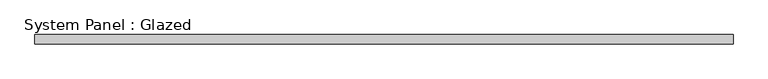
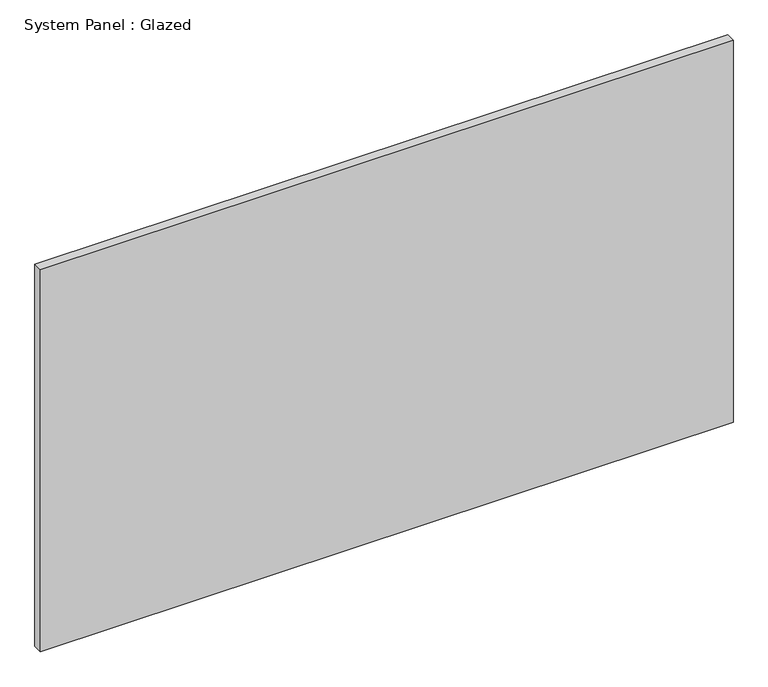
"""IFC4 building model written with IfcOpenShell, lengths in millimetres: plate geometry, System Panel : Glazed."""

from ifc_helpers import new_model, si_unit, origin, origin_with_axes, place, context, project, spatial, polyline, outline, extrude, source, transform, mapped, element, save


def system_panel_glazed_e8634194(model_context):
    return source(origin(), model_context, "Body", "SweptSolid", [
        extrude(outline(polyline([(915.0000002, 24.5), (-915.0000002, 24.5), (-915.0000002, 49.5), (915.0000002, 49.5), (915.0000002, 24.5)])), origin_with_axes(), (0.0, 0.0, 1.0), 1066.8),
    ])


if __name__ == "__main__":
    model = new_model("IFC4")
    model_context = context("Model", 3, world=origin())
    ifc_project = project(units=[si_unit("LENGTHUNIT", "METRE", prefix="MILLI")], contexts=[model_context])
    site = spatial("IfcSite", under=ifc_project)
    building = spatial("IfcBuilding", under=site)
    placement = place(None, origin())
    system_panel_glazed_shape = system_panel_glazed_e8634194(model_context)
    element("IfcPlate", 1, ObjectType="System Panel : Glazed", at=placement, inside=building, context=model_context, shape_type="MappedRepresentation", body=[
        mapped(system_panel_glazed_shape, transform((0.0, 0.0, 0.0), x_axis=(1.0, 0.0, 0.0), y_axis=(0.0, 1.0, 0.0), z_axis=(0.0, 0.0, 1.0))),
    ])
    save(model, "model.ifc")

# Revit data of these elements
# Type "System Panel : Glazed"
#   Keynote = "H11"
#   Construction Type Id = "GSP4R"
#   Analytic Construction = "1/8 in Pilkington single glazing"
#   Visual Light Transmittance = 0.9
#   Solar Heat Gain Coefficient = 0.86
#   Heat Transfer Coefficient (U) = 6.7069 W/(m²·K)
#   Define Thermal Properties by = 1
# Element 1 (IfcPlate, "System Panel : Glazed")
#   Materials on its faces: "Glass"
# Materials
#   "Glass": class "Glass", colour RGB 0 128 192, transparency 0.9, Description = "Soda Lime Glass", Cost = 0
